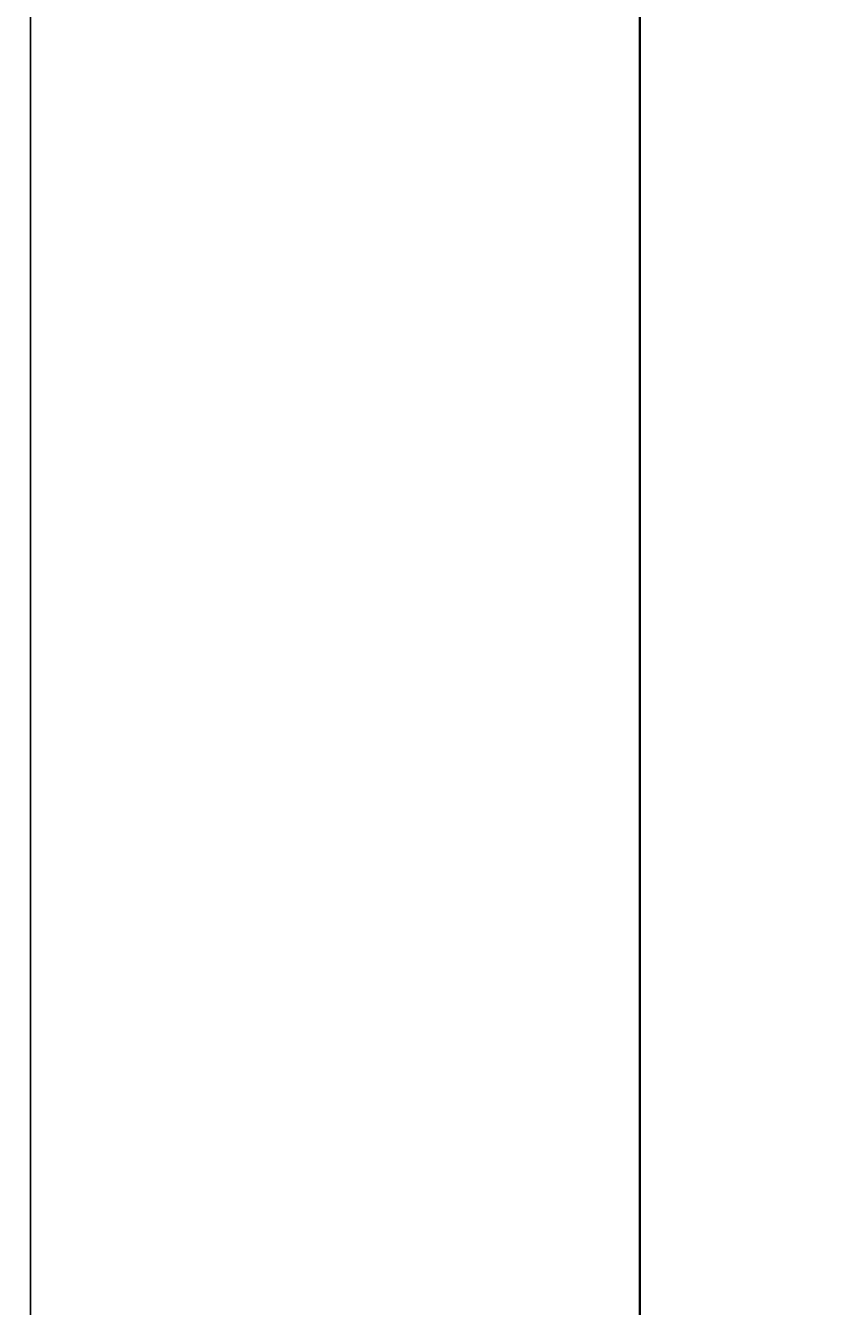
# Model space of a CAD drawing. Units: inches. Extents: x 8049 to 8459, y 820 to 1350.
# Tile 2 of 25: x 8050 to 8083, y 853 to 905. Entities that reach past the tile are written whole.
import ezdxf

# ---------------------------------------------------------------- set-up
doc = ezdxf.new("R2010")
doc.units = ezdxf.units.IN
doc.header["$MEASUREMENT"] = 0
doc.layers.add('A-ANNO-DIMS', color=2, linetype='Continuous', lineweight=18)
doc.layers.add('C-SITE-WALL', color=7, linetype='Continuous', lineweight=35)
doc.styles.get("Standard").update_dxf_attribs({"font": 'arial.ttf'})
doc.dimstyles.get("Standard").update_dxf_attribs({"dimtxt": 0.18, "dimasz": 0.18, "dimexe": 0.18, "dimexo": 0.0625, "dimgap": 0.09, "dimtad": 0, "dimtih": 1, "dimtoh": 1, "dimdec": 4, "dimzin": 0, "dimdsep": 46, "dimtxsty": 'Standard', "dimcen": 0.09, "dimadec": 0, "dimazin": 0, "dimtfac": 1, "dimtdec": 4, "dimtofl": 0, "dimtmove": 0, "dimatfit": 3, "dimfxl": 1, "dimtolj": 1, "dimtzin": 0, "dimarcsym": 0})

# ---------------------------------------------------------------- blocks, each defined once
blk = doc.blocks.new('*D50')
at = {"layer": 'A-ANNO-DIMS', "color": 0, "lineweight": -2, "transparency": 16777216}
for p, q in [((8083.335, 1045.871), (8049.617, 1045.871)), ((8049.797, 1045.691), (8049.797, 945.553)), ((8049.797, 845.051), (8049.797, 945.189)), ((8074.335, 844.871), (8049.617, 844.871))]:
    blk.add_line(p, q, dxfattribs=at)
at = {"layer": 'A-ANNO-DIMS', "color": 0, "transparency": 16777216}
for points in [[(8049.767, 1045.691), (8049.827, 1045.691), (8049.797, 1045.871)], [(8049.767, 845.051), (8049.827, 845.051), (8049.797, 844.871)]]:
    blk.add_solid(points, dxfattribs=at)
at = {"layer": 'Defpoints', "color": 0, "transparency": 16777216}
for p in [(8049.797, 1045.871), (8083.397, 1045.871), (8074.397, 844.871)]:
    blk.add_point(p, dxfattribs=at)
at = {"layer": 'A-ANNO-DIMS', "color": 0, "transparency": 16777216, "insert": (8049.797, 945.371), "char_height": 0.18, "attachment_point": 5}
blk.add_mtext('\\A1;201', dxfattribs=at)

msp = doc.modelspace()

# ---------------------------------------------------------------- linework, layer by layer
at = {"layer": 'C-SITE-WALL'}
msp.add_line((8074.3974, 1324.8706), (8074.3974, 844.8706), dxfattribs=at)

# ---------------------------------------------------------------- dimensions: what is measured, and where the dimension line sits
at = {"layer": 'A-ANNO-DIMS'}
dim = msp.add_linear_dim(base=(8049.7974, 1045.8706), p1=(8074.3974, 844.8706), p2=(8083.3974, 1045.8706), angle=90, dimstyle='Standard', override={"dimdec": 0, "dimlfac": 1, "dimrnd": 0, "dimzin": 0, "dimdsep": 46, "dimlunit": 2}, dxfattribs=at)
dim.commit()
dim.dimension.update_dxf_attribs({"geometry": '*D50', "text_midpoint": (8049.7974, 945.3706)})

doc.saveas('drawing.dxf')
